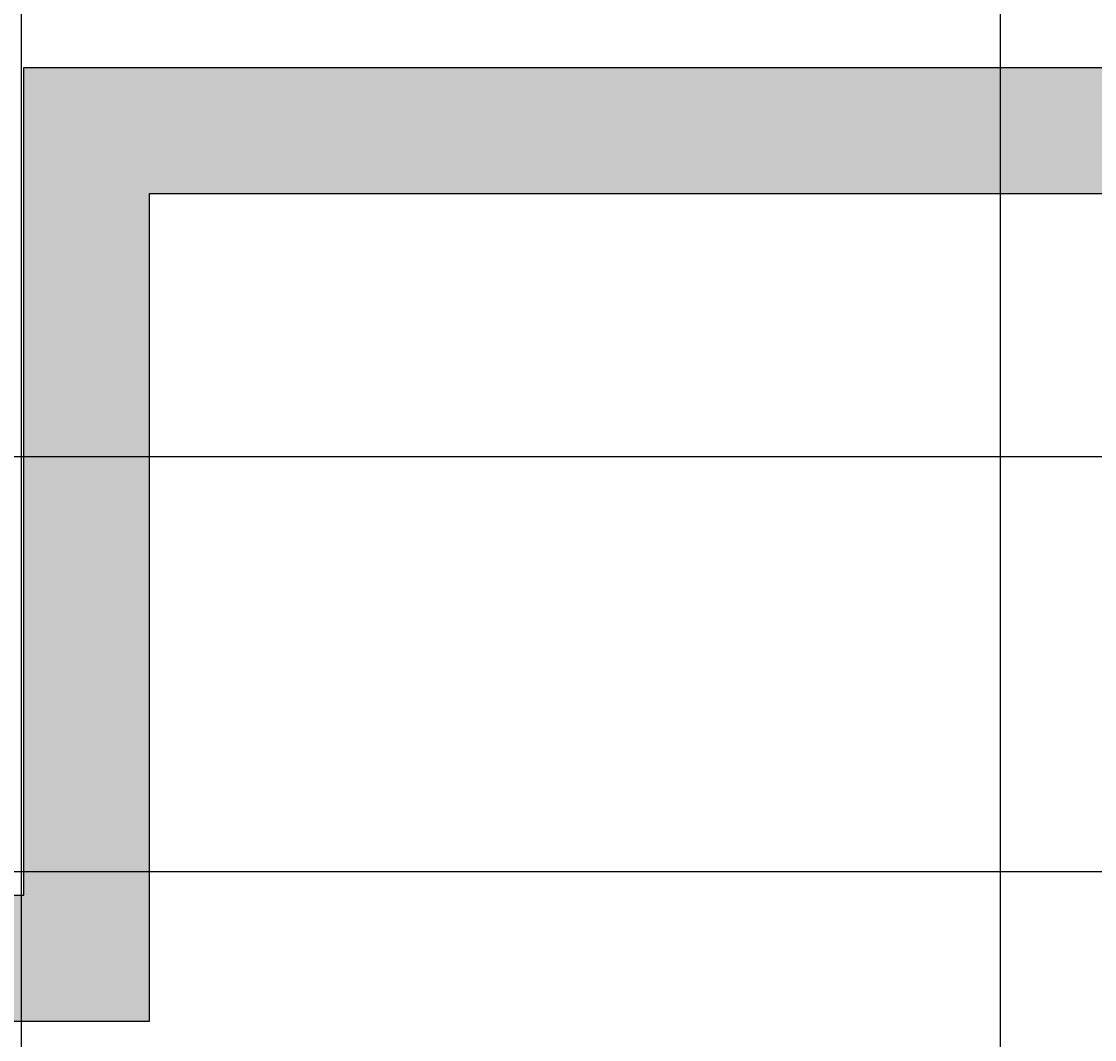
# Model space of a CAD drawing. Units: millimetres. Extents: x -11 to 280, y -4 to 208.
# Tile 42 of 55: x 91 to 121, y 128 to 157. Entities that reach past the tile are written whole.
import ezdxf

# ---------------------------------------------------------------- set-up
doc = ezdxf.new("R2010")
doc.units = ezdxf.units.MM
doc.layers.add('M-DIMS', color=2, linetype='Continuous', lineweight=18)
doc.layers.add('M-HYDR-SUCT', color=7, linetype='Continuous', lineweight=25)
doc.layers.add('M-HYDR-SUCT-PATT', color=221, linetype='Continuous', lineweight=13, true_color=0xff7fdf)
doc.styles.get("Standard").update_dxf_attribs({"font": 'arial.ttf'})
doc.dimstyles.get("Standard").update_dxf_attribs({"dimtxt": 0.18, "dimasz": 0.18, "dimexe": 0.18, "dimexo": 0.0625, "dimgap": 0.09, "dimtad": 0, "dimtih": 1, "dimtoh": 1, "dimdec": 4, "dimzin": 0, "dimdsep": 46, "dimtxsty": 'Standard', "dimcen": 0.09, "dimadec": 0, "dimazin": 0, "dimtfac": 1, "dimtdec": 4, "dimtofl": 0, "dimtmove": 0, "dimatfit": 3, "dimfxl": 1, "dimtolj": 1, "dimtzin": 0, "dimarcsym": 0})

# ---------------------------------------------------------------- blocks, each defined once
blk = doc.blocks.new('*D5')
at = {"layer": 'Defpoints', "color": 0, "transparency": 16777216}
for p in [(24.759, 192.645), (-10.087, 11.435), (261.686, 11.435)]:
    blk.add_point(p, dxfattribs=at)
at = {"layer": 'M-DIMS', "color": 0, "lineweight": -2, "transparency": 16777216}
for p, q in [((24.696, 192.645), (-10.267, 192.645)), ((-10.087, 192.465), (-10.087, 102.222)), ((-10.087, 11.615), (-10.087, 101.858)), ((261.624, 11.435), (-10.267, 11.435))]:
    blk.add_line(p, q, dxfattribs=at)
at = {"layer": 'M-DIMS', "color": 0, "transparency": 16777216}
for points in [[(-10.117, 192.465), (-10.057, 192.465), (-10.087, 192.645)], [(-10.117, 11.615), (-10.057, 11.615), (-10.087, 11.435)]]:
    blk.add_solid(points, dxfattribs=at)
at = {"layer": 'M-DIMS', "color": 0, "transparency": 16777216, "insert": (-10.087, 102.04), "char_height": 0.18, "attachment_point": 5}
blk.add_mtext('\\A1;181.2', dxfattribs=at)
blk = doc.blocks.new('*D11')
at = {"layer": 'Defpoints', "color": 0, "transparency": 16777216}
for p in [(118.514, 207.495), (91.3, 98.149), (118.514, 96.485)]:
    blk.add_point(p, dxfattribs=at)
at = {"layer": 'M-DIMS', "color": 0, "lineweight": -2, "transparency": 16777216}
for p, q in [((91.3, 98.212), (91.3, 207.675)), ((118.514, 96.547), (118.514, 207.675)), ((91.48, 207.495), (104.442, 207.495)), ((118.334, 207.495), (105.372, 207.495))]:
    blk.add_line(p, q, dxfattribs=at)
at = {"layer": 'M-DIMS', "color": 0, "transparency": 16777216}
for points in [[(91.48, 207.525), (91.48, 207.465), (91.3, 207.495)], [(118.334, 207.525), (118.334, 207.465), (118.514, 207.495)]]:
    blk.add_solid(points, dxfattribs=at)
at = {"layer": 'M-DIMS', "color": 0, "transparency": 16777216, "insert": (104.907, 207.495), "char_height": 0.18, "attachment_point": 5}
blk.add_mtext('\\A1;27.214', dxfattribs=at)
blk = doc.blocks.new('*D12')
at = {"layer": 'Defpoints', "color": 0, "transparency": 16777216}
for p in [(173.804, 207.495), (118.514, 96.485), (173.804, 89.387)]:
    blk.add_point(p, dxfattribs=at)
at = {"layer": 'M-DIMS', "color": 0, "lineweight": -2, "transparency": 16777216}
for p, q in [((118.514, 96.547), (118.514, 207.675)), ((173.804, 89.45), (173.804, 207.675)), ((118.694, 207.495), (145.765, 207.495)), ((173.624, 207.495), (146.553, 207.495))]:
    blk.add_line(p, q, dxfattribs=at)
at = {"layer": 'M-DIMS', "color": 0, "transparency": 16777216}
for points in [[(118.694, 207.525), (118.694, 207.465), (118.514, 207.495)], [(173.624, 207.525), (173.624, 207.465), (173.804, 207.495)]]:
    blk.add_solid(points, dxfattribs=at)
at = {"layer": 'M-DIMS', "color": 0, "transparency": 16777216, "insert": (146.159, 207.495), "char_height": 0.18, "attachment_point": 5}
blk.add_mtext('\\A1;55.29', dxfattribs=at)
blk = doc.blocks.new('*D14')
at = {"layer": 'Defpoints', "color": 0, "transparency": 16777216}
for p in [(-10.087, 144.661), (205.531, 144.661), (226.511, 133.123)]:
    blk.add_point(p, dxfattribs=at)
at = {"layer": 'M-DIMS', "color": 0, "lineweight": -2, "transparency": 16777216}
for p, q in [((205.469, 144.661), (-10.267, 144.661)), ((-10.087, 144.481), (-10.087, 139.074)), ((-10.087, 133.303), (-10.087, 138.71)), ((226.448, 133.123), (-10.267, 133.123))]:
    blk.add_line(p, q, dxfattribs=at)
at = {"layer": 'M-DIMS', "color": 0, "transparency": 16777216}
for points in [[(-10.117, 144.481), (-10.057, 144.481), (-10.087, 144.661)], [(-10.117, 133.303), (-10.057, 133.303), (-10.087, 133.123)]]:
    blk.add_solid(points, dxfattribs=at)
at = {"layer": 'M-DIMS', "color": 0, "transparency": 16777216, "insert": (-10.087, 138.892), "char_height": 0.18, "attachment_point": 5}
blk.add_mtext('\\A1;11.538', dxfattribs=at)

msp = doc.modelspace()

# ---------------------------------------------------------------- hatches: boundary and pattern name
at = {"layer": 'M-HYDR-SUCT-PATT'}
h = msp.add_hatch(color=256, dxfattribs=at)
h.set_gradient(color1=(255, 127, 223), color2=(255, 127, 223), tint=1, name='INVCYLINDER')
h.paths.add_polyline_path([(91.3629, 155.4768), (91.3629, 132.4768), (58.3629, 132.4768), (58.3629, 153.9768), (54.8629, 153.9768), (54.8629, 128.9768), (94.8629, 128.9768), (94.8629, 151.9768), (205.5315, 151.9768), (205.5315, 155.4768)])
h.paths.add_polyline_path([(91.3, 114.9452, 1), (78.8273, 114.9452), (78.8273, 108.8141), (42.6453, 108.8141), (42.6453, 153.9768), (39.1453, 153.9768), (39.1453, 105.3141), (78.8273, 105.3141), (78.8273, 98.1491, 1), (91.3, 98.1491), (91.3, 105.3141), (95.5776, 105.3141), (95.5776, 108.8141), (91.3, 108.8141)])
h.paths.add_polyline_path([(228.7, 138.4081), (232.2, 138.4081), (232.2, 144.6609), (228.7, 144.6609)])
h.paths.add_polyline_path([(253.1005, 151.9768, 1), (253.1005, 155.4768), (252.6001, 155.4768), (253.5249, 153.991, -0.1401047), (253.6005, 153.7268, -0.7542249), (252.676, 153.4626), (251.4221, 155.4768), (236.9353, 155.4768), (236.9353, 151.9768)])
h.paths.add_polyline_path([(30.8182, 40.7626), (30.8182, 36.7626), (60.8182, 36.7626), (60.8182, 40.7626)])

# ---------------------------------------------------------------- linework, layer by layer
at = {"layer": 'M-HYDR-SUCT'}
for points in [[(58.3629, 153.9768), (58.3629, 132.4768), (91.3629, 132.4768), (91.3629, 155.4768), (205.5315, 155.4768)], [(54.8629, 153.9768), (54.8629, 128.9768), (94.8629, 128.9768), (94.8629, 151.9768), (205.5315, 151.9768)]]:
    msp.add_lwpolyline(points, dxfattribs=at)

# ---------------------------------------------------------------- dimensions: what is measured, and where the dimension line sits
at = {"layer": 'M-DIMS'}
for base, p1, p2, override, picture, middle in [((118.5137, 207.495), (91.3, 98.1491), (118.5137, 96.4849), {"dimdec": 3, "dimlfac": 1, "dimrnd": 0, "dimzin": 0, "dimdsep": 46, "dimlunit": 2}, '*D11', (104.9068, 207.495)), ((173.8038, 207.495), (118.5137, 96.4849), (173.8038, 89.3873), {"dimdec": 2, "dimlfac": 1, "dimrnd": 0, "dimzin": 0, "dimdsep": 46, "dimlunit": 2}, '*D12', (146.1587, 207.495))]:
    dim = msp.add_linear_dim(base=base, p1=p1, p2=p2, dimstyle='Standard', override=override, dxfattribs=at)
    dim.commit()
    dim.dimension.update_dxf_attribs({"geometry": picture, "text_midpoint": middle})
for base, p1, p2, override, picture, middle in [((-10.0865, 11.4346), (24.7588, 192.645), (261.6863, 11.4346), {"dimdec": 1, "dimlfac": 1, "dimrnd": 0, "dimzin": 0, "dimdsep": 46, "dimlunit": 2}, '*D5', (-10.0865, 102.0398)), ((-10.0865, 144.6609), (226.5106, 133.1228), (205.5315, 144.6609), {"dimdec": 3, "dimlfac": 1, "dimrnd": 0, "dimzin": 0, "dimdsep": 46, "dimlunit": 2}, '*D14', (-10.0865, 138.8918))]:
    dim = msp.add_linear_dim(base=base, p1=p1, p2=p2, angle=90, dimstyle='Standard', override=override, dxfattribs=at)
    dim.commit()
    dim.dimension.update_dxf_attribs({"geometry": picture, "text_midpoint": middle})

doc.saveas('drawing.dxf')
